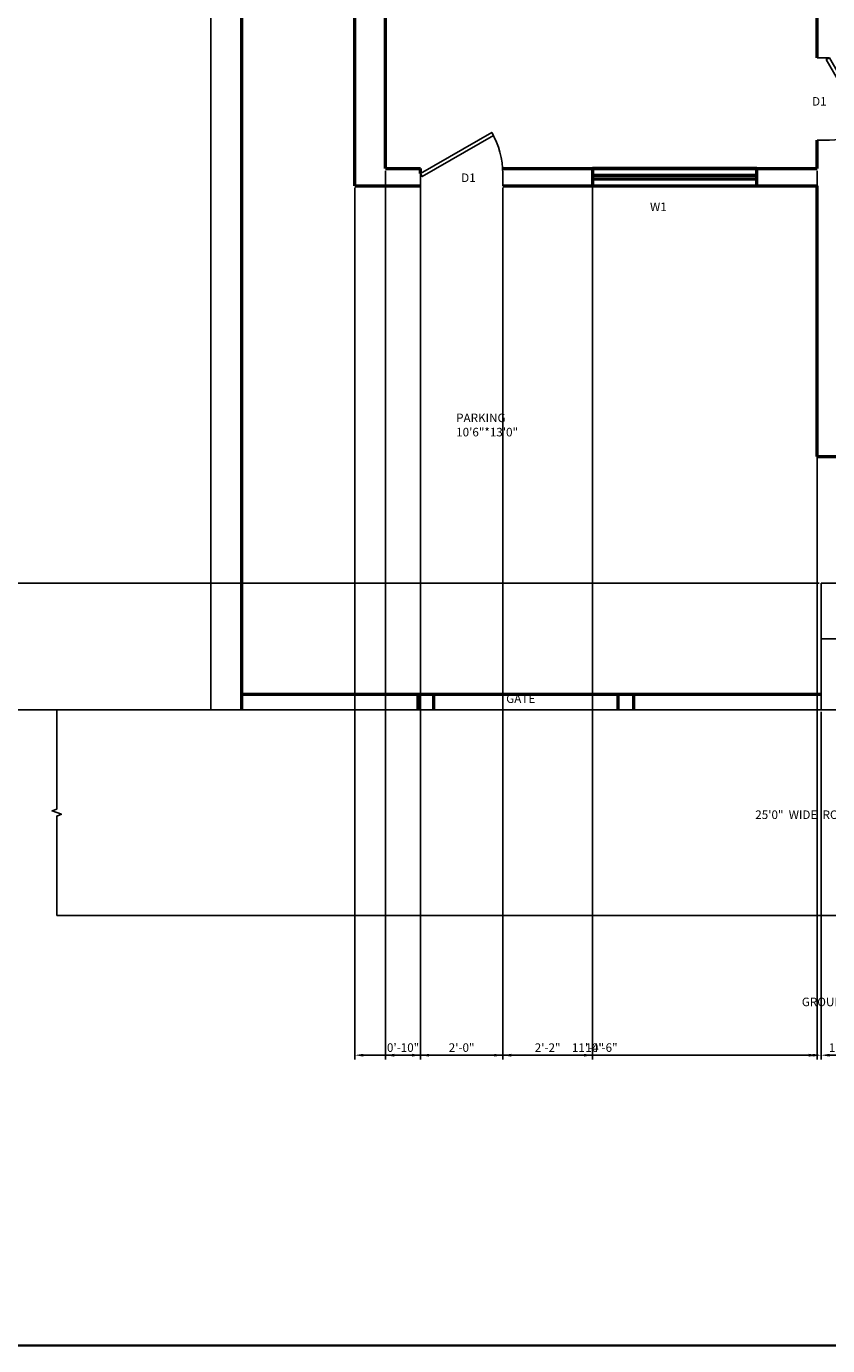
# Model space of a CAD drawing. Units: inches. Extents: x 2020 to 7901, y 1581 to 3943.
# Tile 2 of 17: x 2305 to 2539, y 1581 to 1966. Entities that reach past the tile are written whole.
import ezdxf

# ---------------------------------------------------------------- set-up
doc = ezdxf.new("R2010")
doc.units = ezdxf.units.IN
for name, color, linetype, lineweight in [('A-ANNO-DIMS', 2, 'Continuous', 18), ('A-ANNO-TEXT', 7, 'Continuous', 18), ('A-ANNO-TTLB', 7, 'Continuous', 35), ('A-AREA-IDEN', 3, 'Continuous', 18), ('A-DOOR', 4, 'Continuous', 25), ('A-FLOR-STRS', 3, 'Continuous', 25), ('A-WALL', 7, 'Continuous', 50), ('C-PROP', 6, 'Continuous', 25)]:
    doc.layers.add(name, color=color, linetype=linetype, lineweight=lineweight)
doc.styles.get("Standard").update_dxf_attribs({"font": 'arial.ttf'})
doc.dimstyles.new('ISO-25', dxfattribs={"dimtxt": 2.5, "dimasz": 2.5, "dimexe": 1.25, "dimexo": 0.625, "dimtad": 1, "dimdec": 1, "dimlunit": 3, "dimtxsty": 'Standard', "dimcen": 2.5, "dimadec": 0, "dimazin": 0, "dimtfac": 1, "dimtdec": 1, "dimtmove": 0, "dimatfit": 3, "dimfxl": 1, "dimarcsym": 0})

# ---------------------------------------------------------------- blocks, each defined once
blk = doc.blocks.new('*U2')
for p, q in [((0, 0), (0, -6)), ((40, 0), (40, -6))]:
    blk.add_line(p, q)
blk.add_lwpolyline([(0, 0), (34.64, 20), (35.52, 18.48), (0.87, -1.52)], close=True)
blk.add_arc((0, 0), 40, 0, 30)
blk = doc.blocks.new('*D4')
at = {"layer": 'A-ANNO-DIMS', "color": 0, "lineweight": -2, "transparency": 16777216}
for p, q in [((2358.34, 2246.34), (2285.83, 2246.34)), ((2287.08, 2243.84), (2287.08, 1768.84)), ((2358.34, 1766.34), (2285.83, 1766.34))]:
    blk.add_line(p, q, dxfattribs=at)
at = {"layer": 'A-ANNO-DIMS', "color": 0, "transparency": 16777216}
for points in [[(2286.66, 2243.84), (2287.49, 2243.84), (2287.08, 2246.34)], [(2286.66, 1768.84), (2287.49, 1768.84), (2287.08, 1766.34)]]:
    blk.add_solid(points, dxfattribs=at)
at = {"layer": 'DEFPOINTS', "color": 0, "transparency": 16777216}
for p in [(2358.96, 2246.34), (2287.08, 1766.34), (2358.96, 1766.34)]:
    blk.add_point(p, dxfattribs=at)
at = {"layer": 'A-ANNO-DIMS', "color": 0, "transparency": 16777216, "insert": (2285.18, 2006.34), "char_height": 2.5, "attachment_point": 5, "rotation": 90}
blk.add_mtext("40'", dxfattribs=at)
blk = doc.blocks.new('*D38')
at = {"layer": 'A-ANNO-DIMS', "color": 0, "lineweight": -2, "transparency": 16777216}
for p, q in [((2400.96, 1918.71), (2400.96, 1664.26)), ((2537.1, 1765.71), (2537.1, 1664.26)), ((2403.46, 1665.51), (2534.6, 1665.51))]:
    blk.add_line(p, q, dxfattribs=at)
at = {"layer": 'A-ANNO-DIMS', "color": 0, "transparency": 16777216}
for points in [[(2403.46, 1665.92), (2403.46, 1665.09), (2400.96, 1665.51)], [(2534.6, 1665.92), (2534.6, 1665.09), (2537.1, 1665.51)]]:
    blk.add_solid(points, dxfattribs=at)
at = {"layer": 'DEFPOINTS', "color": 0, "transparency": 16777216}
for p in [(2400.96, 1919.34), (2537.1, 1766.34), (2537.1, 1665.51)]:
    blk.add_point(p, dxfattribs=at)
at = {"layer": 'A-ANNO-DIMS', "color": 0, "transparency": 16777216, "insert": (2469.03, 1667.39), "char_height": 2.5, "attachment_point": 5}
blk.add_mtext('11\'-4"', dxfattribs=at)
blk = doc.blocks.new('*D39')
at = {"layer": 'A-ANNO-DIMS', "color": 0, "lineweight": -2, "transparency": 16777216}
for p, q in [((2537.1, 1765.71), (2537.1, 1664.26)), ((2549.1, 1765.71), (2549.1, 1664.26)), ((2539.6, 1665.51), (2546.6, 1665.51))]:
    blk.add_line(p, q, dxfattribs=at)
at = {"layer": 'A-ANNO-DIMS', "color": 0, "transparency": 16777216}
for points in [[(2539.6, 1665.92), (2539.6, 1665.09), (2537.1, 1665.51)], [(2546.6, 1665.92), (2546.6, 1665.09), (2549.1, 1665.51)]]:
    blk.add_solid(points, dxfattribs=at)
at = {"layer": 'DEFPOINTS', "color": 0, "transparency": 16777216}
for p in [(2537.1, 1766.34), (2549.1, 1766.34), (2549.1, 1665.51)]:
    blk.add_point(p, dxfattribs=at)
at = {"layer": 'A-ANNO-DIMS', "color": 0, "transparency": 16777216, "insert": (2543.1, 1667.41), "char_height": 2.5, "attachment_point": 5}
blk.add_mtext('1\'-0"', dxfattribs=at)
blk = doc.blocks.new('*D42')
at = {"layer": 'A-ANNO-DIMS', "color": 0, "lineweight": -2, "transparency": 16777216}
for p, q in [((2536.48, 1803.34), (2272.67, 1803.34)), ((2273.92, 1768.84), (2273.92, 1800.84)), ((2536.48, 1766.34), (2272.67, 1766.34))]:
    blk.add_line(p, q, dxfattribs=at)
at = {"layer": 'A-ANNO-DIMS', "color": 0, "transparency": 16777216}
for points in [[(2273.5, 1800.84), (2274.33, 1800.84), (2273.92, 1803.34)], [(2273.5, 1768.84), (2274.33, 1768.84), (2273.92, 1766.34)]]:
    blk.add_solid(points, dxfattribs=at)
at = {"layer": 'DEFPOINTS', "color": 0, "transparency": 16777216}
for p in [(2273.92, 1803.34), (2537.1, 1803.34), (2537.1, 1766.34)]:
    blk.add_point(p, dxfattribs=at)
at = {"layer": 'A-ANNO-DIMS', "color": 0, "transparency": 16777216, "insert": (2272.01, 1784.84), "char_height": 2.5, "attachment_point": 5, "rotation": 90}
blk.add_mtext('3\'-1"', dxfattribs=at)
blk = doc.blocks.new('*D101')
at = {"layer": 'A-ANNO-DIMS', "color": 0, "lineweight": -2, "transparency": 16777216}
for p, q in [((2409.96, 1923.71), (2409.96, 1664.26)), ((2535.96, 1923.71), (2535.96, 1664.26)), ((2412.46, 1665.51), (2533.46, 1665.51))]:
    blk.add_line(p, q, dxfattribs=at)
at = {"layer": 'A-ANNO-DIMS', "color": 0, "transparency": 16777216}
for points in [[(2412.46, 1665.92), (2412.46, 1665.09), (2409.96, 1665.51)], [(2533.46, 1665.92), (2533.46, 1665.09), (2535.96, 1665.51)]]:
    blk.add_solid(points, dxfattribs=at)
at = {"layer": 'DEFPOINTS', "color": 0, "transparency": 16777216}
for p in [(2409.96, 1924.34), (2535.96, 1924.34), (2535.96, 1665.51)]:
    blk.add_point(p, dxfattribs=at)
at = {"layer": 'A-ANNO-DIMS', "color": 0, "transparency": 16777216, "insert": (2472.96, 1667.41), "char_height": 2.5, "attachment_point": 5}
blk.add_mtext('10\'-6"', dxfattribs=at)
blk = doc.blocks.new('*D108')
at = {"layer": 'A-ANNO-DIMS', "color": 0, "lineweight": -2, "transparency": 16777216}
for p, q in [((2409.96, 1923.71), (2409.96, 1664.26)), ((2420.14, 1923.71), (2420.14, 1664.26)), ((2412.46, 1665.51), (2417.64, 1665.51))]:
    blk.add_line(p, q, dxfattribs=at)
at = {"layer": 'A-ANNO-DIMS', "color": 0, "transparency": 16777216}
for points in [[(2412.46, 1665.92), (2412.46, 1665.09), (2409.96, 1665.51)], [(2417.64, 1665.92), (2417.64, 1665.09), (2420.14, 1665.51)]]:
    blk.add_solid(points, dxfattribs=at)
at = {"layer": 'DEFPOINTS', "color": 0, "transparency": 16777216}
for p in [(2409.96, 1924.34), (2420.14, 1924.34), (2420.14, 1665.51)]:
    blk.add_point(p, dxfattribs=at)
at = {"layer": 'A-ANNO-DIMS', "color": 0, "transparency": 16777216, "insert": (2415.05, 1667.41), "char_height": 2.5, "attachment_point": 5}
blk.add_mtext('0\'-10"', dxfattribs=at)
blk = doc.blocks.new('*D109')
at = {"layer": 'A-ANNO-DIMS', "color": 0, "lineweight": -2, "transparency": 16777216}
for p, q in [((2420.14, 1918.71), (2420.14, 1664.26)), ((2444.14, 1918.71), (2444.14, 1664.26)), ((2422.64, 1665.51), (2441.64, 1665.51))]:
    blk.add_line(p, q, dxfattribs=at)
at = {"layer": 'A-ANNO-DIMS', "color": 0, "transparency": 16777216}
for points in [[(2422.64, 1665.92), (2422.64, 1665.09), (2420.14, 1665.51)], [(2441.64, 1665.92), (2441.64, 1665.09), (2444.14, 1665.51)]]:
    blk.add_solid(points, dxfattribs=at)
at = {"layer": 'DEFPOINTS', "color": 0, "transparency": 16777216}
for p in [(2420.14, 1919.34), (2444.14, 1919.34), (2444.14, 1665.51)]:
    blk.add_point(p, dxfattribs=at)
at = {"layer": 'A-ANNO-DIMS', "color": 0, "transparency": 16777216, "insert": (2432.14, 1667.41), "char_height": 2.5, "attachment_point": 5}
blk.add_mtext('2\'-0"', dxfattribs=at)
blk = doc.blocks.new('*D110')
at = {"layer": 'A-ANNO-DIMS', "color": 0, "lineweight": -2, "transparency": 16777216}
for p, q in [((2444.14, 1918.71), (2444.14, 1664.26)), ((2470.35, 1918.71), (2470.35, 1664.26)), ((2446.64, 1665.51), (2467.85, 1665.51))]:
    blk.add_line(p, q, dxfattribs=at)
at = {"layer": 'A-ANNO-DIMS', "color": 0, "transparency": 16777216}
for points in [[(2446.64, 1665.92), (2446.64, 1665.09), (2444.14, 1665.51)], [(2467.85, 1665.92), (2467.85, 1665.09), (2470.35, 1665.51)]]:
    blk.add_solid(points, dxfattribs=at)
at = {"layer": 'DEFPOINTS', "color": 0, "transparency": 16777216}
for p in [(2444.14, 1919.34), (2470.35, 1919.34), (2470.35, 1665.51)]:
    blk.add_point(p, dxfattribs=at)
at = {"layer": 'A-ANNO-DIMS', "color": 0, "transparency": 16777216, "insert": (2457.25, 1667.39), "char_height": 2.5, "attachment_point": 5}
blk.add_mtext('2\'-2"', dxfattribs=at)

msp = doc.modelspace()

# ---------------------------------------------------------------- linework, layer by layer
at = {"layer": 'A-ANNO-TTLB'}
msp.add_lwpolyline([(2019.8, 3067.25), (4199.03, 3067.25), (4199.03, 1580.73), (2019.8, 1580.73)], close=True, dxfattribs=at)
at = {"layer": 'A-FLOR-STRS'}
for p, q in [((2537.1, 1803.34), (2537.1, 1766.34)), ((2537.1, 1803.34), (2669.1, 1803.34)), ((2537.1, 1787.09), (2686.94, 1787.09))]:
    msp.add_line(p, q, dxfattribs=at)
at = {"layer": 'A-WALL'}
for p, q in [((2367.96, 1766.34), (2367.96, 2237.34)), ((2400.96, 1919.34), (2400.96, 2173.7)), ((2409.96, 1924.34), (2409.96, 2173.7)), ((2535.96, 1956.67), (2535.96, 2080.34)), ((2535.96, 1924.34), (2535.96, 1932.67)), ((2409.96, 1924.34), (2420.14, 1924.34)), ((2420.14, 1922.9), (2420.14, 1924.34)), ((2444.09, 1924.34), (2535.96, 1924.34)), ((2518.35, 1924.34), (2470.35, 1924.34)), ((2470.35, 1924.34), (2470.35, 1919.34)), ((2518.35, 1922.34), (2470.35, 1922.34)), ((2518.35, 1919.34), (2518.35, 1924.34)), ((2400.96, 1919.34), (2420.14, 1919.34)), ((2444.14, 1919.34), (2535.96, 1919.34)), ((2470.35, 1921.34), (2518.35, 1921.34)), ((2470.35, 1919.34), (2518.35, 1919.34)), ((2535.96, 1840.34), (2535.96, 1919.34)), ((2535.96, 1840.34), (2697.96, 1840.34)), ((2537.1, 1770.84), (2367.96, 1770.84)), ((2419.42, 1766.34), (2419.42, 1770.84)), ((2423.98, 1766.34), (2423.98, 1770.84)), ((2477.82, 1766.34), (2477.82, 1770.84)), ((2482.4, 1766.34), (2482.4, 1770.84))]:
    msp.add_line(p, q, dxfattribs=at)
at = {"layer": 'C-PROP'}
for p, q in [((2358.96, 1766.34), (2358.96, 2246.34)), ((2358.96, 1766.34), (2313.95, 1766.34)), ((2313.95, 1766.34), (2313.95, 1737.34)), ((2718.96, 1766.34), (2358.96, 1766.34)), ((2313.95, 1735.34), (2313.95, 1706.34)), ((2313.95, 1706.34), (2349.95, 1706.34)), ((2349.95, 1706.34), (2718.96, 1706.34))]:
    msp.add_line(p, q, dxfattribs=at)
msp.add_lwpolyline([(2313.95, 1745.26), (2313.95, 1737.34), (2312.57, 1736.84), (2315.32, 1735.84), (2313.95, 1735.34), (2313.95, 1721.57)], dxfattribs=at)

# ---------------------------------------------------------------- block references
at = {"layer": 'A-DOOR', "xscale": 0.6, "yscale": 0.6, "zscale": 0.6, "rotation": 270}
msp.add_blockref('*U2', (2539.5, 1956.67), dxfattribs=at)
at = {"layer": 'A-DOOR', "xscale": 0.6, "yscale": 0.6, "zscale": 0.6}
msp.add_blockref('*U2', (2420.14, 1922.9), dxfattribs=at)

# ---------------------------------------------------------------- texts
at = {"layer": 'A-ANNO-TEXT', "char_height": 2.5, "attachment_point": 1}
for s, width, insert in [('D1', 5.9104, (2534.45, 1945.22)), ('D1', 8.3252, (2432, 1922.92)), ('W1', 17.0851, (2487.13, 1914.43)), ('GATE', 38.0304, (2445.15, 1770.84)), ('25\'0"  WIDE  ROAD', 215.7208, (2517.86, 1736.97)), ('GROUND FLOOR PLAN', 228.0251, (2531.45, 1682.31))]:
    msp.add_mtext_dynamic_manual_height_columns(s, width=width, gutter_width=12.5, heights=[0], dxfattribs=dict(at, insert=insert))
at = {"layer": 'A-AREA-IDEN', "insert": (2430.54, 1852.83), "char_height": 2.5, "attachment_point": 1}
msp.add_mtext_dynamic_manual_height_columns('PARKING\\P10\'6"*13\'0"', width=79.8989, gutter_width=12.5, heights=[0], dxfattribs=at)

# ---------------------------------------------------------------- dimensions: what is measured, and where the dimension line sits
at = {"layer": 'A-ANNO-DIMS'}
for base, p1, p2, override, picture, middle in [((2287.08, 1766.34), (2358.96, 2246.34), (2358.96, 1766.34), {"dimclrd": 0, "dimclre": 0, "dimclrt": 0}, '*D4', (2285.18, 2006.34)), ((2273.92, 1803.34), (2537.1, 1766.34), (2537.1, 1803.34), {"dimdec": 1, "dimlfac": 1, "dimrnd": 0, "dimzin": 1, "dimdsep": 46, "dimlunit": 4, "dimfrac": 2}, '*D42', (2272.01, 1784.84))]:
    dim = msp.add_linear_dim(base=base, p1=p1, p2=p2, angle=90, dimstyle='ISO-25', override=override, dxfattribs=at)
    dim.commit()
    dim.dimension.update_dxf_attribs({"geometry": picture, "text_midpoint": middle})
for base, p1, p2, picture, middle in [((2535.96, 1665.51), (2409.96, 1924.34), (2535.96, 1924.34), '*D101', (2472.96, 1667.41)), ((2420.14, 1665.51), (2409.96, 1924.34), (2420.14, 1924.34), '*D108', (2415.05, 1667.41)), ((2537.1, 1665.51), (2400.96, 1919.34), (2537.1, 1766.34), '*D38', (2469.03, 1667.39)), ((2444.14, 1665.51), (2420.14, 1919.34), (2444.14, 1919.34), '*D109', (2432.14, 1667.41)), ((2470.35, 1665.51), (2444.14, 1919.34), (2470.35, 1919.34), '*D110', (2457.25, 1667.39)), ((2549.1, 1665.51), (2537.1, 1766.34), (2549.1, 1766.34), '*D39', (2543.1, 1667.41))]:
    dim = msp.add_linear_dim(base=base, p1=p1, p2=p2, dimstyle='ISO-25', override={"dimdec": 1, "dimlfac": 1, "dimrnd": 0, "dimzin": 1, "dimdsep": 46, "dimlunit": 4, "dimfrac": 2}, dxfattribs=at)
    dim.commit()
    dim.dimension.update_dxf_attribs({"geometry": picture, "text_midpoint": middle})

doc.saveas('drawing.dxf')
